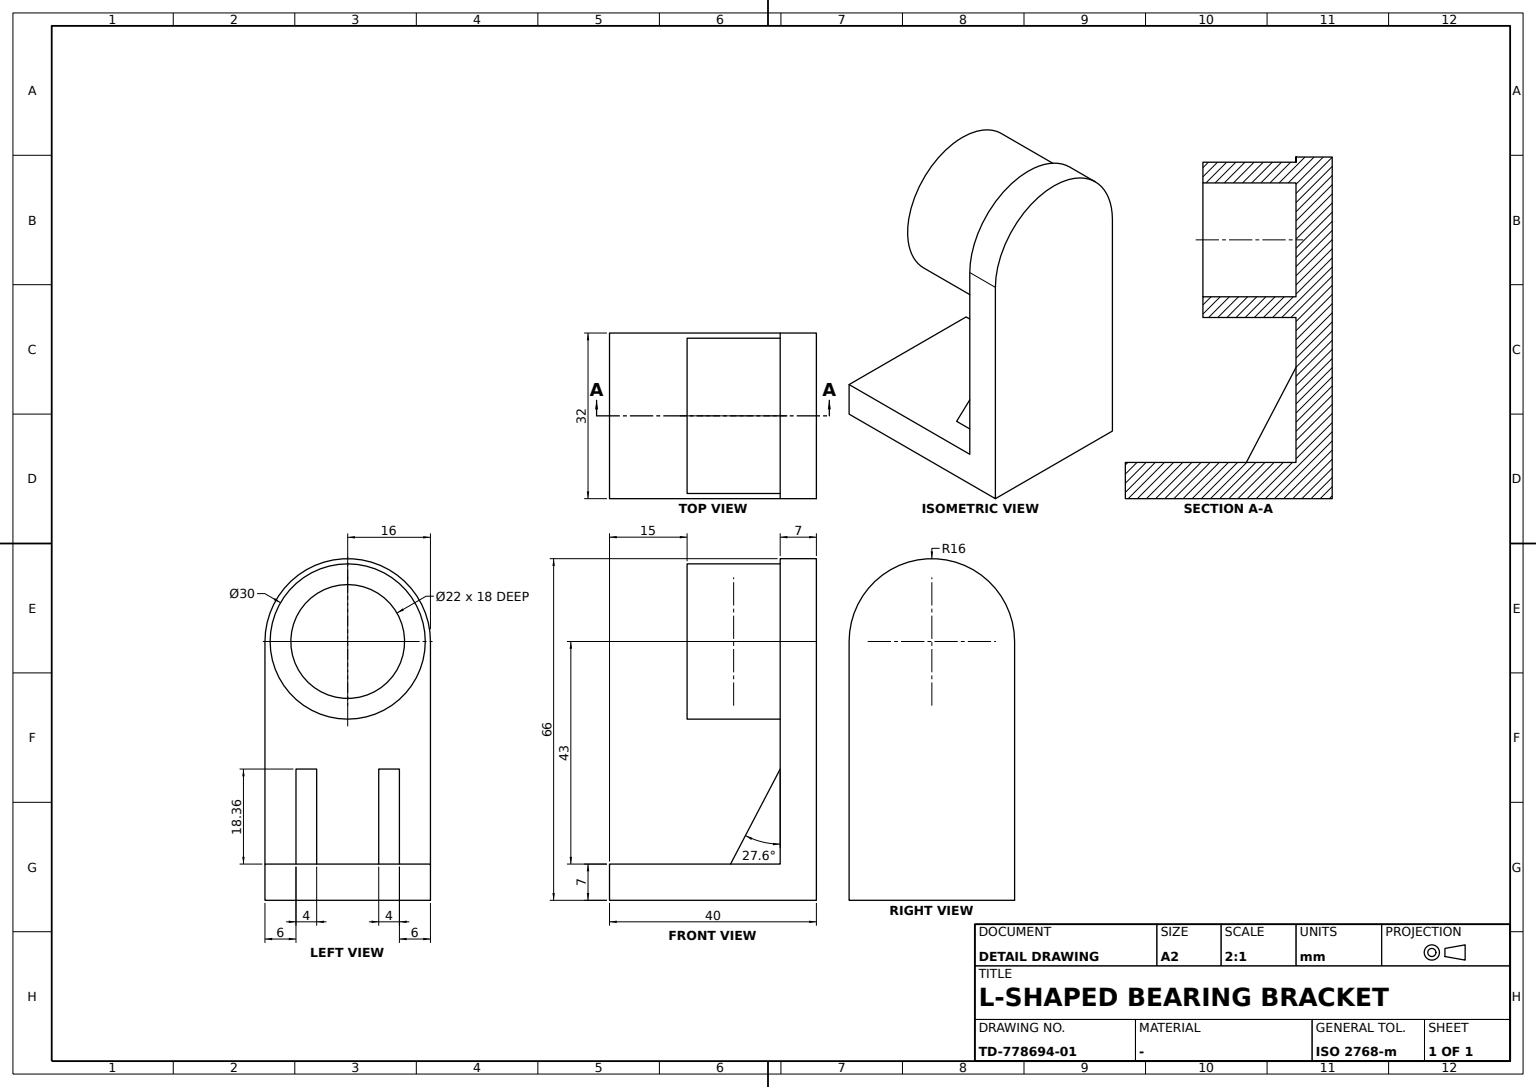
CATIA V5 part; units mm, degrees
sketch "Sketch1" plane through (0, 0, 0) normal (0, 0, 1) x (1, 0, 0)
  line L0 (20, 16) -> (20, -16)
  line L1 (20, -16) -> (-20, -16)
  line L2 (-20, -16) -> (-20, 16)
  line L3 (-20, 16) -> (20, 16)
  dimension "length L0" = 32
  dimension "length L1" = 40
  constraint vertical L0 y-axis
  constraint vertical L2 y-axis
  constraint horizontal L1 x-axis
  constraint horizontal L3 x-axis
  constraint equidistance L0 L2 origin
  constraint equidistance L1 L3 origin
  constraint symmetry L2 L0 y-axis
  constraint symmetry L3 L1 x-axis
extrude "Pad1" add sketch "Sketch1" along normal blind 7
sketch "Sketch2" plane through (20, 0, 0) normal (1, 0, 0) x (0, 1, 0)
  line L0 (-16, 7) -> (16, 7)
  point P0 (0, 50)
  arc A0 (16, 50) -> (-16, 50) centre (0, 50) ccw
  line L1 (16, 7) -> (16, 50)
  line L2 (-16, 7) -> (-16, 50)
  dimension "radius A0" = 16
  dimension "distance L0 P0" = 43
  constraint vertical L1 y-axis
  constraint vertical L2 y-axis
extrude "Pad2" add sketch "Sketch2" against normal blind 7
sketch "Sketch3" plane through (13, 0, 0) normal (-1, 0, 0) x (0, -1, 0)
  line L0 (0, 7) -> (0, 50) construction
  circle A0 centre (0, 50) radius 15
  circle A1 centre (0, 50) radius 11
  dimension "length L0" = 43
  dimension "radius A1" = 11
  dimension "radius A0" = 15
  constraint vertical L0 y-axis
extrude "Pad3" add sketch "Sketch3" along normal blind 18
ref_plane "Plane1" through (0, 10, 0) normal (0, 1, 0) x (-1, 0, 0)
sketch "Sketch4" plane through (0, 10, 0) normal (0, 1, 0) x (-1, 0, 0)
  line L0 (-13, 25.3572) -> (-13, 7)
  line L1 (-13, 7) -> (-3.4014, 7)
  line L2 (-3.4014, 7) -> (-13, 25.3572)
  line L3 (-13, 7) -> (-13, 50) construction
  line L4 (-20, 7) -> (20, 7) construction
  constraint vertical L0 y-axis
  constraint horizontal L1 x-axis
  constraint coincidence L0 L3
  constraint coincidence L1 L4
extrude "Pad4" add sketch "Sketch4" against normal blind 4
mirror "Mirror1" about plane through (0, 0, 0) normal (0, 1, 0)
